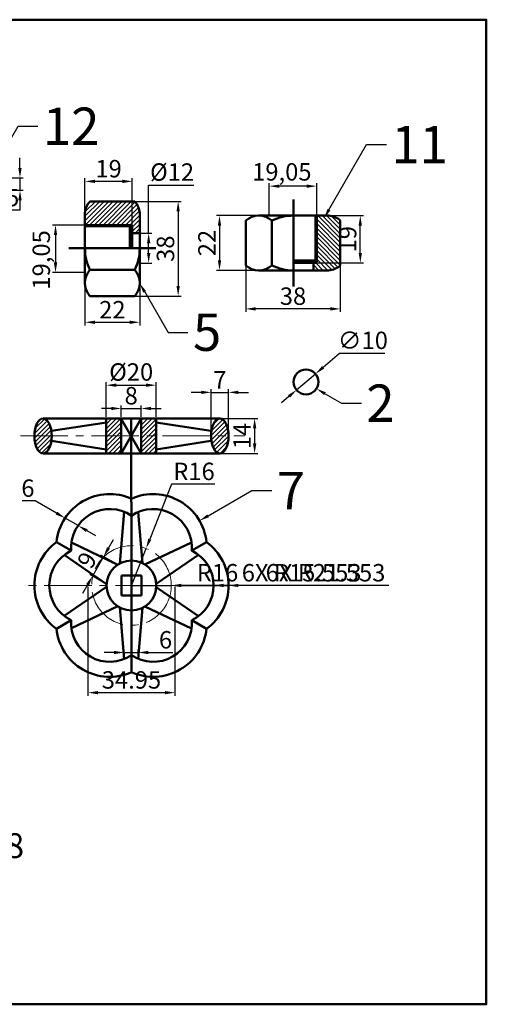
# Model space of a CAD drawing. Units: millimetres. Extents: x 123 to 731, y 468 to 864.
# Tile 5 of 5: x 544 to 731, y 468 to 864. Entities that reach past the tile are written whole.
import ezdxf
from ezdxf import colors
from ezdxf.entities.mleader import LeaderData, LeaderLine
from ezdxf.math import Vec2, Vec3

# ---------------------------------------------------------------- set-up
doc = ezdxf.new("R2010")
doc.units = ezdxf.units.MM
doc.linetypes.add('CENTER2', pattern=[28.575, 19.05, -3.175, 3.175, -3.175])
for name, color, linetype, lineweight in [('M-CNTR', 1, 'CENTER2', 18), ('M-DIMS', 2, 'Continuous', 25), ('M-HATC', 8, 'Continuous', 18), ('M-OUTL', 7, 'Continuous', 50), ('M-TEXT', 3, 'Continuous', 25)]:
    doc.layers.add(name, color=color, linetype=linetype, lineweight=lineweight)
doc.styles.get("Standard").update_dxf_attribs({"font": 'arial.ttf'})
doc.dimstyles.new('ISO-25', dxfattribs={"dimtxt": 7, "dimasz": 4, "dimexe": 1.25, "dimexo": 0.625, "dimtad": 1, "dimtoh": 1, "dimtxsty": 'Standard', "dimcen": 2.5, "dimadec": 0, "dimazin": 0, "dimtfac": 1, "dimtmove": 0, "dimatfit": 3, "dimfxl": 1, "dimarcsym": 0})

# ---------------------------------------------------------------- blocks, each defined once
blk = doc.blocks.new('*D51')
at = {"layer": 'Defpoints', "color": 0, "transparency": 16777216}
for p in [(535.28, 800.43), (531.28, 795.43), (544.03, 795.43)]:
    blk.add_point(p, dxfattribs=at)
at = {"layer": 'M-DIMS', "color": 0, "lineweight": -2, "transparency": 16777216}
for p, q in [((544.03, 804.43), (544.03, 808.43)), ((535.9, 800.43), (545.28, 800.43)), ((544.03, 800.43), (544.03, 795.43)), ((531.9, 795.43), (545.28, 795.43)), ((544.03, 791.43), (544.03, 787.43)), ((544.03, 787.43), (538.76, 787.43))]:
    blk.add_line(p, q, dxfattribs=at)
at = {"layer": 'M-DIMS', "color": 0, "transparency": 16777216}
for points in [[(543.36, 804.43), (544.69, 804.43), (544.03, 800.43)], [(543.36, 791.43), (544.69, 791.43), (544.03, 795.43)]]:
    blk.add_solid(points, dxfattribs=at)
at = {"layer": 'M-DIMS', "color": 0, "transparency": 16777216, "insert": (541.08, 791.61), "char_height": 7, "attachment_point": 5}
blk.add_mtext('5', dxfattribs=at)
blk = doc.blocks.new('*D61')
at = {"layer": 'Defpoints', "color": 0, "transparency": 16777216}
for p in [(570.15, 799.01), (589.15, 779.89), (570.15, 778.96)]:
    blk.add_point(p, dxfattribs=at)
at = {"layer": 'M-DIMS', "color": 0, "lineweight": -2, "transparency": 16777216}
for p, q in [((570.15, 779.58), (570.15, 800.26)), ((585.15, 799.01), (574.15, 799.01)), ((589.15, 780.52), (589.15, 800.26))]:
    blk.add_line(p, q, dxfattribs=at)
at = {"layer": 'M-DIMS', "color": 0, "transparency": 16777216}
for points in [[(574.15, 799.68), (574.15, 798.34), (570.15, 799.01)], [(585.15, 799.68), (585.15, 798.34), (589.15, 799.01)]]:
    blk.add_solid(points, dxfattribs=at)
at = {"layer": 'M-DIMS', "color": 0, "transparency": 16777216, "insert": (579.65, 803.21), "char_height": 7, "attachment_point": 5}
blk.add_mtext('19', dxfattribs=at)
blk = doc.blocks.new('*D62')
at = {"layer": 'Defpoints', "color": 0, "transparency": 16777216}
for p in [(570.15, 781.49), (558.31, 762.44), (570.15, 762.44)]:
    blk.add_point(p, dxfattribs=at)
at = {"layer": 'M-DIMS', "color": 0, "lineweight": -2, "transparency": 16777216}
for p, q in [((569.52, 781.49), (557.06, 781.49)), ((558.31, 777.49), (558.31, 766.44)), ((569.52, 762.44), (557.06, 762.44))]:
    blk.add_line(p, q, dxfattribs=at)
at = {"layer": 'M-DIMS', "color": 0, "transparency": 16777216}
for points in [[(557.65, 777.49), (558.98, 777.49), (558.31, 781.49)], [(557.65, 766.44), (558.98, 766.44), (558.31, 762.44)]]:
    blk.add_solid(points, dxfattribs=at)
at = {"layer": 'M-DIMS', "color": 0, "transparency": 16777216, "insert": (553.48, 767.47), "char_height": 7, "attachment_point": 5, "rotation": 90}
blk.add_mtext('19,05', dxfattribs=at)
blk = doc.blocks.new('*D63')
at = {"layer": 'Defpoints', "color": 0, "transparency": 16777216}
for p in [(570.15, 758.07), (592.15, 758.29), (592.15, 742.41)]:
    blk.add_point(p, dxfattribs=at)
at = {"layer": 'M-DIMS', "color": 0, "lineweight": -2, "transparency": 16777216}
for p, q in [((570.15, 757.44), (570.15, 741.16)), ((592.15, 757.67), (592.15, 741.16)), ((574.15, 742.41), (588.15, 742.41))]:
    blk.add_line(p, q, dxfattribs=at)
at = {"layer": 'M-DIMS', "color": 0, "transparency": 16777216}
for points in [[(574.15, 743.08), (574.15, 741.75), (570.15, 742.41)], [(588.15, 743.08), (588.15, 741.75), (592.15, 742.41)]]:
    blk.add_solid(points, dxfattribs=at)
at = {"layer": 'M-DIMS', "color": 0, "transparency": 16777216, "insert": (581.15, 746.55), "char_height": 7, "attachment_point": 5}
blk.add_mtext('22', dxfattribs=at)
blk = doc.blocks.new('*D64')
at = {"layer": 'Defpoints', "color": 0, "transparency": 16777216}
for p in [(581.15, 790.96), (581.15, 752.96), (607.61, 752.96)]:
    blk.add_point(p, dxfattribs=at)
at = {"layer": 'M-DIMS', "color": 0, "lineweight": -2, "transparency": 16777216}
for p, q in [((581.78, 790.96), (608.86, 790.96)), ((607.61, 786.96), (607.61, 756.96)), ((581.78, 752.96), (608.86, 752.96))]:
    blk.add_line(p, q, dxfattribs=at)
at = {"layer": 'M-DIMS', "color": 0, "transparency": 16777216}
for points in [[(606.94, 786.96), (608.27, 786.96), (607.61, 790.96)], [(606.94, 756.96), (608.27, 756.96), (607.61, 752.96)]]:
    blk.add_solid(points, dxfattribs=at)
at = {"layer": 'M-DIMS', "color": 0, "transparency": 16777216, "insert": (603.41, 771.96), "char_height": 7, "attachment_point": 5, "rotation": 90}
blk.add_mtext('38', dxfattribs=at)
blk = doc.blocks.new('*D65')
at = {"layer": 'Defpoints', "color": 0, "transparency": 16777216}
for p in [(592.15, 778.18), (592.15, 766.18), (595.75, 766.18)]:
    blk.add_point(p, dxfattribs=at)
at = {"layer": 'M-DIMS', "color": 0, "lineweight": -2, "transparency": 16777216}
for p, q in [((595.75, 778.18), (595.75, 797.46)), ((595.75, 797.46), (613.95, 797.46)), ((592.78, 778.18), (597, 778.18)), ((595.75, 770.18), (595.75, 774.18)), ((592.78, 766.18), (597, 766.18))]:
    blk.add_line(p, q, dxfattribs=at)
at = {"layer": 'M-DIMS', "color": 0, "transparency": 16777216}
for points in [[(595.09, 774.18), (596.42, 774.18), (595.75, 778.18)], [(595.09, 770.18), (596.42, 770.18), (595.75, 766.18)]]:
    blk.add_solid(points, dxfattribs=at)
at = {"layer": 'M-DIMS', "color": 0, "transparency": 16777216, "insert": (605.16, 801.85), "char_height": 7, "attachment_point": 5}
blk.add_mtext('%%C12', dxfattribs=at)
blk = doc.blocks.new('*D67')
at = {"layer": 'Defpoints', "color": 0, "transparency": 16777216}
for p in [(660.76, 785.26), (680.82, 785.26), (661.7, 766.26)]:
    blk.add_point(p, dxfattribs=at)
at = {"layer": 'M-DIMS', "color": 0, "lineweight": -2, "transparency": 16777216}
for p, q in [((661.39, 785.26), (682.07, 785.26)), ((680.82, 770.26), (680.82, 781.26)), ((662.32, 766.26), (682.07, 766.26))]:
    blk.add_line(p, q, dxfattribs=at)
at = {"layer": 'M-DIMS', "color": 0, "transparency": 16777216}
for points in [[(680.15, 781.26), (681.48, 781.26), (680.82, 785.26)], [(680.15, 770.26), (681.48, 770.26), (680.82, 766.26)]]:
    blk.add_solid(points, dxfattribs=at)
at = {"layer": 'M-DIMS', "color": 0, "transparency": 16777216, "insert": (676.62, 775.76), "char_height": 7, "attachment_point": 5, "rotation": 90}
blk.add_mtext('19', dxfattribs=at)
blk = doc.blocks.new('*D66')
at = {"layer": 'Defpoints', "color": 0, "transparency": 16777216}
for p in [(644.24, 797.1), (644.24, 785.26), (663.29, 785.26)]:
    blk.add_point(p, dxfattribs=at)
at = {"layer": 'M-DIMS', "color": 0, "lineweight": -2, "transparency": 16777216}
for p, q in [((644.24, 785.88), (644.24, 798.35)), ((659.29, 797.1), (648.24, 797.1)), ((663.29, 785.88), (663.29, 798.35))]:
    blk.add_line(p, q, dxfattribs=at)
at = {"layer": 'M-DIMS', "color": 0, "transparency": 16777216}
for points in [[(648.24, 797.76), (648.24, 796.43), (644.24, 797.1)], [(659.29, 797.76), (659.29, 796.43), (663.29, 797.1)]]:
    blk.add_solid(points, dxfattribs=at)
at = {"layer": 'M-DIMS', "color": 0, "transparency": 16777216, "insert": (649.28, 801.93), "char_height": 7, "attachment_point": 5}
blk.add_mtext('19,05', dxfattribs=at)
blk = doc.blocks.new('*D68')
at = {"layer": 'Defpoints', "color": 0, "transparency": 16777216}
for p in [(639.87, 785.26), (624.22, 763.26), (640.1, 763.26)]:
    blk.add_point(p, dxfattribs=at)
at = {"layer": 'M-DIMS', "color": 0, "lineweight": -2, "transparency": 16777216}
for p, q in [((639.25, 785.26), (622.97, 785.26)), ((624.22, 781.26), (624.22, 767.26)), ((639.47, 763.26), (622.97, 763.26))]:
    blk.add_line(p, q, dxfattribs=at)
at = {"layer": 'M-DIMS', "color": 0, "transparency": 16777216}
for points in [[(623.55, 781.26), (624.88, 781.26), (624.22, 785.26)], [(623.55, 767.26), (624.88, 767.26), (624.22, 763.26)]]:
    blk.add_solid(points, dxfattribs=at)
at = {"layer": 'M-DIMS', "color": 0, "transparency": 16777216, "insert": (620.08, 774.26), "char_height": 7, "attachment_point": 5, "rotation": 90}
blk.add_mtext('22', dxfattribs=at)
blk = doc.blocks.new('*D69')
at = {"layer": 'Defpoints', "color": 0, "transparency": 16777216}
for p in [(634.77, 774.26), (672.77, 774.26), (634.77, 747.8)]:
    blk.add_point(p, dxfattribs=at)
at = {"layer": 'M-DIMS', "color": 0, "lineweight": -2, "transparency": 16777216}
for p, q in [((634.77, 773.63), (634.77, 746.55)), ((672.77, 773.63), (672.77, 746.55)), ((668.77, 747.8), (638.77, 747.8))]:
    blk.add_line(p, q, dxfattribs=at)
at = {"layer": 'M-DIMS', "color": 0, "transparency": 16777216}
for points in [[(638.77, 748.47), (638.77, 747.13), (634.77, 747.8)], [(668.77, 748.47), (668.77, 747.13), (672.77, 747.8)]]:
    blk.add_solid(points, dxfattribs=at)
at = {"layer": 'M-DIMS', "color": 0, "transparency": 16777216, "insert": (653.77, 752), "char_height": 7, "attachment_point": 5}
blk.add_mtext('38', dxfattribs=at)
blk = doc.blocks.new('*U82')
at = {"layer": 'M-CNTR', "color": 0, "transparency": 16777216}
blk.add_line((-53.48, 0), (36.6, 0), dxfattribs=at)
blk = doc.blocks.new('*D84')
at = {"layer": 'Defpoints', "color": 0, "transparency": 16777216}
for p in [(598.73, 717.14), (578.73, 703.75), (598.73, 703.75)]:
    blk.add_point(p, dxfattribs=at)
at = {"layer": 'M-DIMS', "color": 0, "lineweight": -2, "transparency": 16777216}
for p, q in [((578.73, 704.38), (578.73, 718.39)), ((582.73, 717.14), (594.73, 717.14)), ((598.73, 704.38), (598.73, 718.39))]:
    blk.add_line(p, q, dxfattribs=at)
at = {"layer": 'M-DIMS', "color": 0, "transparency": 16777216}
for points in [[(582.73, 717.81), (582.73, 716.47), (578.73, 717.14)], [(594.73, 717.81), (594.73, 716.47), (598.73, 717.14)]]:
    blk.add_solid(points, dxfattribs=at)
at = {"layer": 'M-DIMS', "color": 0, "transparency": 16777216, "insert": (588.73, 721.54), "char_height": 7, "attachment_point": 5}
blk.add_mtext('%%C20', dxfattribs=at)
blk = doc.blocks.new('*D85')
at = {"layer": 'Defpoints', "color": 0, "transparency": 16777216}
for p in [(592.73, 707.8), (584.73, 703.75), (592.73, 703.75)]:
    blk.add_point(p, dxfattribs=at)
at = {"layer": 'M-DIMS', "color": 0, "lineweight": -2, "transparency": 16777216}
for p, q in [((584.73, 704.38), (584.73, 709.05)), ((592.73, 704.38), (592.73, 709.05)), ((580.73, 707.8), (576.73, 707.8)), ((584.73, 707.8), (592.73, 707.8)), ((596.73, 707.8), (600.73, 707.8))]:
    blk.add_line(p, q, dxfattribs=at)
at = {"layer": 'M-DIMS', "color": 0, "transparency": 16777216}
for points in [[(580.73, 708.46), (580.73, 707.13), (584.73, 707.8)], [(596.73, 708.46), (596.73, 707.13), (592.73, 707.8)]]:
    blk.add_solid(points, dxfattribs=at)
at = {"layer": 'M-DIMS', "color": 0, "transparency": 16777216, "insert": (588.73, 712), "char_height": 7, "attachment_point": 5}
blk.add_mtext('8', dxfattribs=at)
blk = doc.blocks.new('*D86')
at = {"layer": 'Defpoints', "color": 0, "transparency": 16777216}
for p in [(627.86, 714.26), (620.86, 696.75), (627.86, 696.75)]:
    blk.add_point(p, dxfattribs=at)
at = {"layer": 'M-DIMS', "color": 0, "lineweight": -2, "transparency": 16777216}
for p, q in [((616.86, 714.26), (612.86, 714.26)), ((620.86, 697.38), (620.86, 715.51)), ((620.86, 714.26), (627.86, 714.26)), ((627.86, 697.38), (627.86, 715.51)), ((631.86, 714.26), (635.86, 714.26))]:
    blk.add_line(p, q, dxfattribs=at)
at = {"layer": 'M-DIMS', "color": 0, "transparency": 16777216}
for points in [[(616.86, 714.93), (616.86, 713.59), (620.86, 714.26)], [(631.86, 714.93), (631.86, 713.59), (627.86, 714.26)]]:
    blk.add_solid(points, dxfattribs=at)
at = {"layer": 'M-DIMS', "color": 0, "transparency": 16777216, "insert": (624.36, 718.38), "char_height": 7, "attachment_point": 5}
blk.add_mtext('7', dxfattribs=at)
blk = doc.blocks.new('*D87')
at = {"layer": 'Defpoints', "color": 0, "transparency": 16777216}
for p in [(615.05, 703.75), (615.05, 689.75), (638.35, 689.75)]:
    blk.add_point(p, dxfattribs=at)
at = {"layer": 'M-DIMS', "color": 0, "lineweight": -2, "transparency": 16777216}
for p, q in [((615.67, 703.75), (639.6, 703.75)), ((638.35, 699.75), (638.35, 693.75)), ((615.67, 689.75), (639.6, 689.75))]:
    blk.add_line(p, q, dxfattribs=at)
at = {"layer": 'M-DIMS', "color": 0, "transparency": 16777216}
for points in [[(637.68, 699.75), (639.02, 699.75), (638.35, 703.75)], [(637.68, 693.75), (639.02, 693.75), (638.35, 689.75)]]:
    blk.add_solid(points, dxfattribs=at)
at = {"layer": 'M-DIMS', "color": 0, "transparency": 16777216, "insert": (634.21, 696.75), "char_height": 7, "attachment_point": 5, "rotation": 90}
blk.add_mtext('14', dxfattribs=at)
blk = doc.blocks.new('*D88')
at = {"layer": 'Defpoints', "color": 0, "transparency": 16777216}
for p in [(562.43, 664.18), (567.4, 660.72), (567.65, 661.17)]:
    blk.add_point(p, dxfattribs=at)
at = {"layer": 'M-DIMS', "color": 0, "lineweight": -2, "transparency": 16777216}
for p, q in [((550.15, 670.68), (544.9, 670.68)), ((558.71, 665.74), (550.15, 670.68)), ((562.12, 663.64), (561.55, 662.66)), ((567.4, 660.72), (562.18, 663.74)), ((567.34, 660.62), (566.77, 659.64)), ((570.86, 658.72), (574.33, 656.72))]:
    blk.add_line(p, q, dxfattribs=at)
at = {"layer": 'M-DIMS', "color": 0, "transparency": 16777216}
for points in [[(559.04, 666.32), (558.38, 665.16), (562.18, 663.74)], [(571.2, 659.3), (570.53, 658.15), (567.4, 660.72)]]:
    blk.add_solid(points, dxfattribs=at)
at = {"layer": 'M-DIMS', "color": 0, "transparency": 16777216, "insert": (547.21, 674.88), "char_height": 7, "attachment_point": 5}
blk.add_mtext('6', dxfattribs=at)
blk = doc.blocks.new('*D89')
at = {"layer": 'Defpoints', "color": 0, "transparency": 16777216}
for p in [(594.73, 651.57), (588.83, 636.7)]:
    blk.add_point(p, dxfattribs=at)
at = {"layer": 'M-DIMS', "color": 0, "lineweight": -2, "transparency": 16777216}
for p, q in [((604.99, 677.41), (596.21, 655.29)), ((622.33, 677.41), (604.99, 677.41)), ((588.83, 636.7), (594.73, 651.57))]:
    blk.add_line(p, q, dxfattribs=at)
at = {"layer": 'M-DIMS', "color": 0, "transparency": 16777216}
blk.add_solid([(595.59, 655.54), (596.83, 655.04), (594.73, 651.57)], dxfattribs=at)
at = {"layer": 'M-DIMS', "color": 0, "transparency": 16777216, "insert": (613.97, 681.61), "char_height": 7, "attachment_point": 5}
blk.add_mtext('R16', dxfattribs=at)
blk = doc.blocks.new('*D90')
at = {"layer": 'Defpoints', "color": 0, "transparency": 16777216}
for p in [(591.59, 609.77), (585.86, 607.12), (591.59, 607.21)]:
    blk.add_point(p, dxfattribs=at)
at = {"layer": 'M-DIMS', "color": 0, "lineweight": -2, "transparency": 16777216}
for p, q in [((581.86, 609.77), (577.86, 609.77)), ((585.86, 607.75), (585.86, 611.02)), ((585.86, 609.77), (591.59, 609.77)), ((591.59, 607.83), (591.59, 611.02)), ((595.59, 609.77), (605.47, 609.77))]:
    blk.add_line(p, q, dxfattribs=at)
at = {"layer": 'M-DIMS', "color": 0, "transparency": 16777216}
for points in [[(581.86, 610.44), (581.86, 609.11), (585.86, 609.77)], [(595.59, 610.44), (595.59, 609.11), (591.59, 609.77)]]:
    blk.add_solid(points, dxfattribs=at)
at = {"layer": 'M-DIMS', "color": 0, "transparency": 16777216, "insert": (602.53, 613.97), "char_height": 7, "attachment_point": 5}
blk.add_mtext('6', dxfattribs=at)
blk = doc.blocks.new('*D91')
at = {"layer": 'Defpoints', "color": 0, "transparency": 16777216}
for p in [(583.31, 645.04), (573.17, 640.44), (578.85, 637.2)]:
    blk.add_point(p, dxfattribs=at)
at = {"layer": 'M-DIMS', "color": 0, "lineweight": -2, "transparency": 16777216}
for p, q in [((579.61, 651.74), (581.59, 655.22)), ((582.77, 645.35), (576.55, 648.89)), ((577.63, 648.27), (573.17, 640.44)), ((578.3, 637.51), (572.08, 641.05)), ((571.19, 636.96), (569.21, 633.48))]:
    blk.add_line(p, q, dxfattribs=at)
at = {"layer": 'M-DIMS', "color": 0, "transparency": 16777216}
for points in [[(579.03, 652.07), (580.19, 651.41), (577.63, 648.27)], [(570.61, 637.29), (571.77, 636.63), (573.17, 640.44)]]:
    blk.add_solid(points, dxfattribs=at)
at = {"layer": 'M-DIMS', "color": 0, "transparency": 16777216, "insert": (571.75, 646.43), "char_height": 7, "attachment_point": 5, "rotation": 60.3324}
blk.add_mtext('9', dxfattribs=at)
blk = doc.blocks.new('*D92')
at = {"layer": 'Defpoints', "color": 0, "transparency": 16777216}
for p in [(662.81, 721.7), (655.19, 715.22)]:
    blk.add_point(p, dxfattribs=at)
at = {"layer": 'M-DIMS', "color": 0, "lineweight": -2, "transparency": 16777216}
for p, q in [((672.41, 729.86), (665.86, 724.29)), ((690.66, 729.86), (672.41, 729.86)), ((655.19, 715.22), (662.81, 721.7)), ((652.14, 712.63), (649.09, 710.04))]:
    blk.add_line(p, q, dxfattribs=at)
at = {"layer": 'M-DIMS', "color": 0, "transparency": 16777216}
for points in [[(665.43, 724.8), (666.29, 723.78), (662.81, 721.7)], [(651.71, 713.14), (652.57, 712.13), (655.19, 715.22)]]:
    blk.add_solid(points, dxfattribs=at)
at = {"layer": 'M-DIMS', "color": 0, "transparency": 16777216, "insert": (681.85, 734.25), "char_height": 7, "attachment_point": 5}
blk.add_mtext('∅10', dxfattribs=at)
blk = doc.blocks.new('*D95')
at = {"layer": 'Defpoints', "color": 0, "transparency": 16777216}
for p in [(571.36, 636.7), (606.31, 636.7), (606.31, 593.64)]:
    blk.add_point(p, dxfattribs=at)
at = {"layer": 'M-DIMS', "color": 0, "lineweight": -2, "transparency": 16777216}
for p, q in [((571.36, 636.08), (571.36, 592.39)), ((606.31, 636.08), (606.31, 592.39)), ((575.36, 593.64), (602.31, 593.64))]:
    blk.add_line(p, q, dxfattribs=at)
at = {"layer": 'M-DIMS', "color": 0, "transparency": 16777216}
for points in [[(575.36, 594.31), (575.36, 592.98), (571.36, 593.64)], [(602.31, 594.31), (602.31, 592.98), (606.31, 593.64)]]:
    blk.add_solid(points, dxfattribs=at)
at = {"layer": 'M-DIMS', "color": 0, "transparency": 16777216, "insert": (588.83, 597.85), "char_height": 7, "attachment_point": 5}
blk.add_mtext('34.95', dxfattribs=at)
blk = doc.blocks.new('*D98')
at = {"layer": 'Defpoints', "color": 0, "transparency": 16777216}
for p in [(606.31, 636.7), (627.86, 636.7)]:
    blk.add_point(p, dxfattribs=at)
at = {"layer": 'M-DIMS', "color": 0, "lineweight": -2, "transparency": 16777216}
for p, q in [((606.31, 636.7), (627.86, 636.7)), ((640.79, 636.7), (631.86, 636.7)), ((692.26, 636.7), (640.79, 636.7))]:
    blk.add_line(p, q, dxfattribs=at)
at = {"layer": 'M-DIMS', "color": 0, "transparency": 16777216}
blk.add_solid([(631.86, 637.37), (631.86, 636.03), (627.86, 636.7)], dxfattribs=at)
at = {"layer": 'M-DIMS', "color": 0, "transparency": 16777216, "insert": (666.84, 640.9), "char_height": 7, "attachment_point": 5}
blk.add_mtext('6X R21.553', dxfattribs=at)
blk = doc.blocks.new('*D99')
at = {"layer": 'Defpoints', "color": 0, "transparency": 16777216}
for p in [(606.31, 636.7), (621.86, 636.7)]:
    blk.add_point(p, dxfattribs=at)
at = {"layer": 'M-DIMS', "color": 0, "lineweight": -2, "transparency": 16777216}
for p, q in [((606.31, 636.7), (621.86, 636.7)), ((631.19, 636.7), (625.86, 636.7)), ((682.66, 636.7), (631.19, 636.7))]:
    blk.add_line(p, q, dxfattribs=at)
at = {"layer": 'M-DIMS', "color": 0, "transparency": 16777216}
blk.add_solid([(625.86, 637.37), (625.86, 636.03), (621.86, 636.7)], dxfattribs=at)
at = {"layer": 'M-DIMS', "color": 0, "transparency": 16777216, "insert": (657.24, 640.9), "char_height": 7, "attachment_point": 5}
blk.add_mtext('6X R15.553', dxfattribs=at)
blk = doc.blocks.new('*D100')
at = {"layer": 'Defpoints', "color": 0, "transparency": 16777216}
for p in [(588.83, 636.7), (604.83, 636.7)]:
    blk.add_point(p, dxfattribs=at)
at = {"layer": 'M-DIMS', "color": 0, "lineweight": -2, "transparency": 16777216}
for p, q in [((588.83, 636.7), (604.83, 636.7)), ((614.43, 636.7), (608.83, 636.7)), ((631.78, 636.7), (614.43, 636.7))]:
    blk.add_line(p, q, dxfattribs=at)
at = {"layer": 'M-DIMS', "color": 0, "transparency": 16777216}
blk.add_solid([(608.83, 637.37), (608.83, 636.03), (604.83, 636.7)], dxfattribs=at)
at = {"layer": 'M-DIMS', "color": 0, "transparency": 16777216, "insert": (623.42, 640.9), "char_height": 7, "attachment_point": 5}
blk.add_mtext('R16', dxfattribs=at)

msp = doc.modelspace()

# ---------------------------------------------------------------- hatches: boundary and pattern name
at = {"layer": 'M-HATC'}
h = msp.add_hatch(dxfattribs=at)
h.set_pattern_fill('ANSI31', color=256, scale=0.4)
h.set_pattern_definition([(45, (-43.1623, -15.1066), (-0.8980256, 0.8980256), [])])
h.paths.add_polyline_path([(572.1506, 790.9613, 0.16687276), (570.1506, 786.287), (570.1506, 781.4863), (588.6506, 781.4863, -0.41421356), (589.1506, 780.9863), (589.1506, 778.1776), (592.1506, 778.1776), (592.1506, 786.287, 0.16687276), (590.1506, 790.9613)])
h = msp.add_hatch(dxfattribs=at)
h.set_pattern_fill('ANSI31', color=256, scale=0.4, angle=-90)
h.set_pattern_definition([(315, (-118.1955, 1427.0609), (0.8980256, 0.8980256), [])])
h.paths.add_polyline_path([(672.7658, 783.2581, 0.16687276), (668.0915, 785.2581), (663.2908, 785.2581), (663.2908, 766.7581, -0.41421356), (662.7908, 766.2581), (661.9821, 766.2581), (661.9821, 763.2581), (668.0915, 763.2581, 0.16687276), (672.7658, 765.2581)])
h = msp.add_hatch(dxfattribs=at)
h.set_pattern_fill('ANSI31', color=256, scale=0.4)
h.set_pattern_definition([(45, (-66.3643, -11.869), (-0.8980256, 0.8980256), [])])
edge = h.paths.add_edge_path()
edge.add_ellipse((553.3058, 696.7534), major_axis=(0, -7), ratio=0.5, start_angle=90, end_angle=270)
edge.add_line((549.8058, 696.7534), (556.8058, 696.7534))
edge = h.paths.add_edge_path()
edge.add_ellipse((553.3058, 696.7534), major_axis=(0, -7), ratio=0.5, start_angle=270, end_angle=450)
edge.add_line((556.8058, 696.7534), (549.8058, 696.7534))
h.paths.add_polyline_path([(584.7251, 703.7534), (578.7251, 703.7534), (578.7251, 696.7534), (584.7251, 696.7534)])
h.paths.add_polyline_path([(584.7251, 696.7534), (578.7251, 696.7534), (578.7251, 689.7534), (584.7251, 689.7534)])
h.paths.add_polyline_path([(598.7251, 703.7534), (592.7251, 703.7534), (592.7251, 696.7534), (598.7251, 696.7534)])
h.paths.add_polyline_path([(592.7251, 696.7534), (592.7251, 689.7534), (598.7251, 689.7534), (598.7251, 696.7534)])
edge = h.paths.add_edge_path()
edge.add_ellipse((624.3605, 696.7534), major_axis=(0, -7), ratio=0.5, start_angle=90, end_angle=270)
edge.add_line((620.8605, 696.7534), (627.8605, 696.7534))
edge = h.paths.add_edge_path()
edge.add_ellipse((624.3605, 696.7534), major_axis=(0, -7), ratio=0.5, start_angle=270, end_angle=450)
edge.add_line((627.8605, 696.7534), (620.8605, 696.7534))

# ---------------------------------------------------------------- linework, layer by layer
at = {"layer": 'M-CNTR'}
msp.add_line((630.0003, 636.7006), (547.4498, 636.7006), dxfattribs=at)
msp.add_circle((588.8332, 636.7006), 16, dxfattribs=at)
at = {"layer": 'M-OUTL'}
for p, q in [((653.9821, 791.7301), (653.9821, 756.7417)), ((590.1506, 790.9613), (572.1506, 790.9613)), ((570.1506, 786.287), (570.1506, 758.0681)), ((592.1506, 758.0681), (592.1506, 786.287)), ((634.7658, 783.2581), (634.7658, 765.2581)), ((668.0915, 785.2581), (639.8726, 785.2581)), ((645.2658, 783.2581), (645.2658, 765.2581)), ((653.7658, 785.2581), (663.2908, 785.2581)), ((662.7908, 767.2581), (662.7908, 785.2581)), ((663.2908, 785.2581), (663.2908, 766.7581)), ((672.7658, 765.2581), (672.7658, 783.2581)), ((570.1506, 771.9613), (570.1506, 781.4863)), ((570.1506, 781.4863), (588.6506, 781.4863)), ((588.1506, 780.9863), (570.1506, 780.9863)), ((588.1506, 780.9863), (588.1506, 772.1776)), ((589.1506, 780.9863), (589.1506, 772.1776)), ((589.1506, 778.1776), (592.1506, 778.1776)), ((563.6786, 772.1776), (598.6671, 772.1776)), ((572.1506, 763.4613), (590.1506, 763.4613)), ((662.7908, 767.2581), (653.9821, 767.2581)), ((662.7908, 766.2581), (653.9821, 766.2581)), ((661.9821, 763.2581), (661.9821, 766.2581)), ((639.8726, 763.2581), (668.0915, 763.2581)), ((653.9821, 763.2581), (661.9821, 763.2581)), ((572.1506, 752.9613), (590.1506, 752.9613)), ((553.3058, 703.7534), (624.3605, 703.7534)), ((556.6689, 698.7541), (578.7494, 702.1264)), ((578.7251, 689.7534), (578.7251, 703.7534)), ((584.7251, 689.7534), (584.7251, 703.7534)), ((584.7251, 689.7534), (592.7251, 703.7534)), ((592.7251, 689.7534), (584.7251, 703.6099)), ((588.8332, 636.7006), (588.7251, 703.7534)), ((592.7251, 689.7534), (592.7251, 703.7534)), ((620.7812, 698.7541), (598.7007, 702.1264)), ((598.7251, 689.7534), (598.7251, 703.7534)), ((556.6599, 694.7534), (578.7251, 691.2818)), ((620.7902, 694.7534), (598.7251, 691.2818)), ((588.7251, 689.7534), (553.3058, 689.7534)), ((624.3605, 689.7534), (588.7251, 689.7534)), ((584.2251, 645.5756), (585.8636, 666.2778)), ((593.2251, 645.6846), (591.5945, 666.1929)), ((558.6645, 654.1185), (564.5845, 650.7006)), ((583.3081, 645.0358), (564.6812, 653.9021)), ((594.2757, 645.0899), (612.972, 653.9974)), ((613.0819, 650.7006), (619.0018, 654.1185)), ((578.8457, 637.202), (561.7721, 648.9476)), ((598.813, 637.3352), (615.7937, 649.0257)), ((584.8332, 640.7006), (592.8332, 640.7006)), ((584.8332, 632.7006), (584.8332, 640.7006)), ((592.8332, 640.7006), (592.8332, 632.7006)), ((578.8452, 636.2094), (561.771, 624.4545)), ((588.8332, 608.7006), (588.8332, 636.7006)), ((598.8124, 636.0561), (615.7927, 624.3748)), ((592.8332, 632.7006), (584.8332, 632.7006)), ((583.2997, 628.3711), (564.681, 619.5006)), ((584.216, 627.8304), (585.8624, 607.123)), ((593.2161, 627.7123), (591.5933, 607.2089)), ((594.2554, 628.3116), (612.9719, 619.4026)), ((558.6645, 619.2828), (564.5845, 622.7006)), ((613.0819, 622.7006), (619.0018, 619.2828)), ((588.8332, 608.7006), (588.8332, 601.8649))]:
    msp.add_line(p, q, dxfattribs=at)
msp.add_lwpolyline([(123.3719, 863.9604), (731.4761, 863.9604), (731.4761, 468.4518), (123.3719, 468.4518)], close=True, dxfattribs=at)
for points in [[(619.0018, 619.2828, 0.50859868), (619.0018, 654.1185, 0.50859868), (588.8332, 671.5364, 0.50859868), (558.6645, 654.1185, 0.50859868), (558.6645, 619.2828, 0.50859868), (588.8332, 601.8649, 0.50859868)], [(613.0819, 622.7006, 0.62704729), (613.0819, 650.7006, 0.62704729), (588.8332, 664.7006, 0.62704729), (564.5845, 650.7006, 0.62704729), (564.5845, 622.7006, 0.62704729), (588.8332, 608.7006, 0.62704729)]]:
    msp.add_lwpolyline(points, format="xyb", close=True, dxfattribs=at)
for centre, radius in [((658.9986, 718.4612), 5), ((588.8332, 636.7006), 10)]:
    msp.add_circle(centre, radius, dxfattribs=at)
for centre, radius, start, end in [((577.9584, 785.7113), 7.829, 137.887598, 175.782841), ((584.3429, 785.7113), 7.829, 4.217159, 42.112402), ((640.0158, 777.3726), 7.8868, 48.266285, 131.733715), ((653.7658, 766.1956), 19.0625, 89.350067, 116.48104), ((667.5158, 777.4503), 7.829, 47.887598, 85.782841), ((588.6506, 780.9863), 0.5, 0, 180), ((589.2131, 771.9613), 19.0625, 179.350067, 206.48104), ((573.0881, 771.9613), 19.0625, 333.51896, 0.649933), ((578.0361, 758.2113), 7.8868, 138.266285, 221.733715), ((584.2651, 758.2113), 7.8868, 318.266285, 41.733715), ((640.0158, 771.1436), 7.8868, 228.266285, 311.733715), ((653.7658, 782.3206), 19.0625, 243.51896, 270.649933), ((662.7908, 766.7581), 0.5, 270, 90), ((667.5158, 771.0659), 7.829, 274.217159, 312.112402), ((588.8332, 636.7006), 28, 90, 90.221233)]:
    msp.add_arc(centre, radius, start, end, dxfattribs=at)
for centre in [(553.3058, 696.7534), (624.3605, 696.7534)]:
    msp.add_ellipse(centre, major_axis=(0, -7), ratio=0.5, dxfattribs=at)

# ---------------------------------------------------------------- block references
at = {"layer": 'M-CNTR'}
msp.add_blockref('*U82', (597.688, 696.7534), dxfattribs=at)

# ---------------------------------------------------------------- dimensions: what is measured, and where the dimension line sits
at = {"layer": 'M-DIMS'}
for base, p1, p2, angle, picture, middle in [((544.027, 795.4278), (535.2797, 800.4278), (531.2797, 795.4278), 90, '*D51', (541.0814, 791.6125)), ((624.2171, 763.2572), (639.8726, 785.2581), (640.0959, 763.2572), 270, '*D68', (620.0777, 774.2577)), ((680.8152, 785.2581), (661.6966, 766.2581), (660.76, 785.2581), 270, '*D67', (676.6162, 775.7581)), ((638.3511, 689.7534), (615.0481, 703.7534), (615.0481, 689.7534), 90, '*D87', (634.2118, 696.7534))]:
    dim = msp.add_linear_dim(base=base, p1=p1, p2=p2, angle=angle, dimstyle='ISO-25', override={"dimclrd": 0, "dimclre": 0, "dimclrt": 0}, dxfattribs=at)
    dim.commit()
    dim.dimension.update_dxf_attribs({"geometry": picture, "text_midpoint": middle})
for base, p1, p2, override, picture, middle in [((570.1506, 799.0107), (589.1506, 779.8921), (570.1506, 778.9555), {"dimclrd": 0, "dimclre": 0, "dimclrt": 0}, '*D61', (579.6506, 803.2097)), ((592.1515, 742.4126), (570.1506, 758.0681), (592.1515, 758.2914), {"dimclrd": 0, "dimclre": 0, "dimclrt": 0}, '*D63', (581.1511, 746.5519)), ((627.8605, 714.2598), (620.8605, 696.7534), (627.8605, 696.7534), {"dimclrd": 0, "dimclre": 0, "dimclrt": 0}, '*D86', (624.3605, 718.3848)), ((592.7251, 707.7969), (584.7251, 703.7534), (592.7251, 703.7534), {"dimclrd": 0, "dimclre": 0, "dimclrt": 0}, '*D85', (588.7251, 711.9959)), ((606.3078, 593.6448), (571.3586, 636.7006), (606.3078, 636.7006), {"dimdec": 2, "dimlfac": 1, "dimrnd": 0, "dimzin": 0, "dimdsep": 46, "dimlunit": 2}, '*D95', (588.8332, 597.8462))]:
    dim = msp.add_linear_dim(base=base, p1=p1, p2=p2, dimstyle='ISO-25', override=override, dxfattribs=at)
    dim.commit()
    dim.dimension.update_dxf_attribs({"geometry": picture, "text_midpoint": middle})
for base, p1, p2, angle, text, picture, middle, dimtype in [((595.7534, 766.1776), (592.1506, 778.1776), (592.1506, 766.1776), 90, '%%C<>', '*D65', (605.1642, 797.4571), 160), ((567.3982, 660.7235), (562.4303, 664.1811), (567.6534, 661.1655), 330, '6', '*D88', (547.2112, 670.6833), 161)]:
    dim = msp.add_linear_dim(base=base, p1=p1, p2=p2, angle=angle, text=text, dimstyle='ISO-25', override={"dimclrd": 0, "dimclre": 0, "dimclrt": 0}, dxfattribs=at)
    dim.commit()
    dim.dimension.update_dxf_attribs({"geometry": picture, "text_midpoint": middle, "dimtype": dimtype})
for base, p1, p2, picture, middle in [((644.2408, 797.0952), (663.2908, 785.2594), (644.2408, 785.2594), '*D66', (649.2792, 797.0952)), ((634.7658, 747.801), (672.7658, 774.2581), (634.7658, 774.2581), '*D69', (653.7658, 747.801))]:
    dim = msp.add_linear_dim(base=base, p1=p1, p2=p2, dimstyle='ISO-25', override={"dimclrd": 0, "dimclre": 0, "dimclrt": 0}, dxfattribs=at)
    dim.commit()
    dim.dimension.update_dxf_attribs({"geometry": picture, "text_midpoint": middle, "dimtype": 160})
for base, p1, p2, picture, middle in [((607.6077, 752.9613), (581.1506, 790.9613), (581.1506, 752.9613), '*D64', (607.6077, 771.9613)), ((558.3136, 762.4363), (570.1493, 781.4863), (570.1493, 762.4363), '*D62', (558.3136, 767.4747))]:
    dim = msp.add_linear_dim(base=base, p1=p1, p2=p2, angle=90, dimstyle='ISO-25', override={"dimclrd": 0, "dimclre": 0, "dimclrt": 0}, dxfattribs=at)
    dim.commit()
    dim.dimension.update_dxf_attribs({"geometry": picture, "text_midpoint": middle, "dimtype": 160})
dim = msp.add_diameter_dim_2p(p1=(655.1882, 715.2238), p2=(662.8091, 721.6986), dimstyle='ISO-25', override={"dimclrd": 0, "dimclre": 0, "dimclrt": 0}, dxfattribs=at)
dim.commit()
dim.dimension.update_dxf_attribs({"geometry": '*D92', "text_midpoint": (681.8482, 729.8586), "dimtype": 163})
for base, p1, p2, text, picture, middle in [((598.7251, 717.1415), (578.7251, 703.7534), (598.7251, 703.7534), '%%C<>', '*D84', (588.7251, 721.5363)), ((591.5933, 609.7747), (585.8624, 607.123), (591.5933, 607.2089), '6', '*D90', (602.5293, 613.9737))]:
    dim = msp.add_linear_dim(base=base, p1=p1, p2=p2, text=text, dimstyle='ISO-25', override={"dimclrd": 0, "dimclre": 0, "dimclrt": 0}, dxfattribs=at)
    dim.commit()
    dim.dimension.update_dxf_attribs({"geometry": picture, "text_midpoint": middle})
for mpoint, override, picture, middle in [((594.734, 651.5728), {"dimclrd": 0, "dimclre": 0, "dimclrt": 0}, '*D89', (613.9725, 677.4126)), ((604.8332, 636.701), {"dimdec": 0, "dimlfac": 1, "dimrnd": 0, "dimzin": 0, "dimdsep": 46, "dimlunit": 2}, '*D100', (614.4332, 636.7012))]:
    dim = msp.add_radius_dim(center=(588.8332, 636.7006), mpoint=mpoint, dimstyle='ISO-25', override=override, dxfattribs=at)
    dim.commit()
    dim.dimension.update_dxf_attribs({"geometry": picture, "text_midpoint": middle, "dimtype": 164})
dim = msp.add_aligned_dim(p1=(583.3081, 645.0358), p2=(578.8457, 637.202), distance=-6.5327, text='9', dimstyle='ISO-25', override={"dimclrd": 0, "dimclre": 0, "dimclrt": 0}, dxfattribs=at)
dim.commit()
dim.dimension.update_dxf_attribs({"geometry": '*D91', "text_midpoint": (571.752, 646.4308)})
for mpoint, picture, middle in [((627.8605, 636.701), '*D98', (640.7922, 636.7012)), ((621.8605, 636.701), '*D99', (631.1922, 636.7012))]:
    dim = msp.add_radius_dim(center=(606.3078, 636.7006), mpoint=mpoint, text='6X <>', dimstyle='ISO-25', override={"dimdec": 3, "dimlfac": 1, "dimrnd": 0, "dimzin": 0, "dimdsep": 46, "dimlunit": 2}, dxfattribs=at)
    dim.commit()
    dim.dimension.update_dxf_attribs({"geometry": picture, "text_midpoint": middle, "dimtype": 164})

# ---------------------------------------------------------------- leaders
at = {"layer": 'M-TEXT'}
ml = msp.add_multileader_mtext('Standard', dxfattribs=at)
ml.set_content('12', color=256)
ml.set_leader_properties()
ml.build(insert=Vec2(0, 0))
ctx = ml.context
ctx.base_point, ctx.char_height, ctx.plane_origin = Vec3(551.2554, 821.1704), 15, Vec3(531.2797, 800.4278)
notes = []
notes.append((ctx, [(0, (1, 1, 0), (543.2554, 821.1704), (1, 0), 8, [(0, [(531.2797, 800.4278)], 0, [])])]))
ctx.mtext.insert, ctx.mtext.flow_direction = Vec3(553.2554, 828.6704), 5
ml = msp.add_multileader_mtext('Standard', dxfattribs=at)
ml.set_content('11', color=256)
ml.set_leader_properties()
ml.build(insert=Vec2(0, 0))
ctx = ml.context
ctx.base_point, ctx.char_height, ctx.plane_origin = Vec3(691.3258, 813.7986), 15, Vec3(666.2261, 784.1811)
notes.append((ctx, [(0, (1, 1, 0), (683.3258, 813.7986), (1, 0), 8, [(0, [(666.2261, 784.1811)], 0, [])])]))
ctx.mtext.insert, ctx.mtext.flow_direction = Vec3(693.3258, 821.2986), 5
ml = msp.add_multileader_mtext('Standard', dxfattribs=at)
ml.set_content('5', color=256)
ml.set_leader_properties()
ml.build(insert=Vec2(0, 0))
ctx = ml.context
ctx.base_point, ctx.char_height, ctx.plane_origin = Vec3(611.5595, 738.3073), 15, Vec3(592.1506, 758.0681)
notes.append((ctx, [(0, (1, 1, 0), (603.5595, 738.3073), (1, 0), 8, [(0, [(592.1506, 758.0681)], 0, [])])]))
ctx.mtext.insert, ctx.mtext.flow_direction = Vec3(613.5595, 745.9352), 5
ml = msp.add_multileader_mtext('Standard', dxfattribs=at)
ml.set_content('2', color=256)
ml.set_leader_properties()
ml.build(insert=Vec2(0, 0))
ctx = ml.context
ctx.base_point, ctx.char_height, ctx.plane_origin = Vec3(681.2376, 709.9235), 15, Vec3(663.185, 715.7273)
notes.append((ctx, [(0, (1, 1, 0), (673.2376, 709.9235), (1, 0), 8, [(0, [(663.185, 715.7273)], 0, [])])]))
ctx.mtext.insert, ctx.mtext.flow_direction = Vec3(683.2376, 717.4235), 5
ml = msp.add_multileader_mtext('Standard', dxfattribs=at)
ml.set_content('7', color=256)
ml.set_leader_properties()
ml.build(insert=Vec2(0, 0))
ctx = ml.context
ctx.base_point, ctx.char_height, ctx.plane_origin = Vec3(645.2577, 674.8377), 15, Vec3(616.1965, 662.6781)
notes.append((ctx, [(0, (1, 1, 0), (637.2577, 674.8377), (1, 0), 8, [(0, [(616.1965, 662.6781)], 0, [])])]))
ctx.mtext.insert, ctx.mtext.flow_direction = Vec3(647.2577, 682.3377), 5
ml = msp.add_multileader_mtext('Standard', dxfattribs=at)
ml.set_content('8', color=256)
ml.set_leader_properties()
ml.build(insert=Vec2(0, 0))
ctx = ml.context
ctx.base_point, ctx.char_height, ctx.plane_origin = Vec3(536.1336, 532.1043), 10, Vec3(518.0866, 541.0375)
notes.append((ctx, [(0, (1, 1, 0), (528.1336, 532.1043), (1, 0), 8, [(0, [(518.0866, 541.0375)], 0, [])])]))
ctx.mtext.insert, ctx.mtext.flow_direction = Vec3(538.1336, 537.1896), 5
for ctx, leaders in notes:
    for number, flags, end, landing, length, lines in leaders:
        leader = LeaderData()
        leader.index, (leader.has_last_leader_line, leader.has_dogleg_vector, leader.attachment_direction) = number, flags
        leader.last_leader_point, leader.dogleg_vector, leader.dogleg_length = Vec3(end), Vec3(landing), length
        for number, points, colour, breaks in lines:
            line = LeaderLine()
            line.index, line.vertices, line.color, line.breaks = number, Vec3.list(points), colors.encode_raw_color(colour), breaks
            leader.lines.append(line)
        ctx.leaders.append(leader)

doc.saveas('drawing.dxf')
